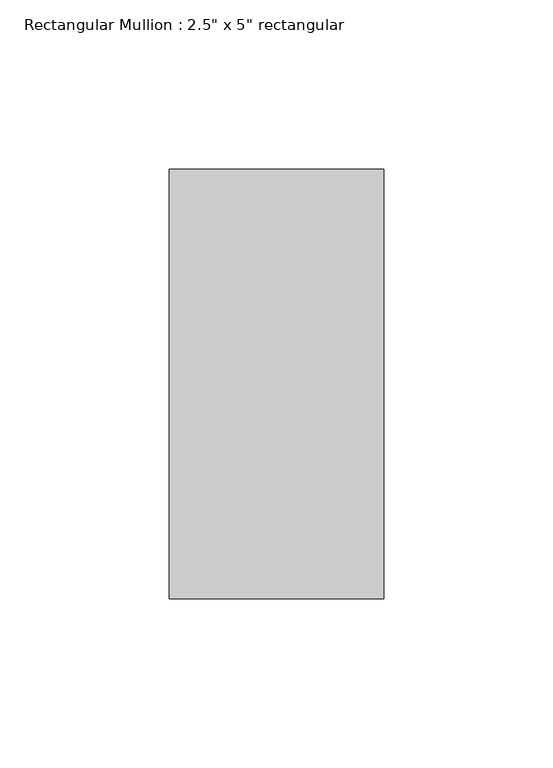
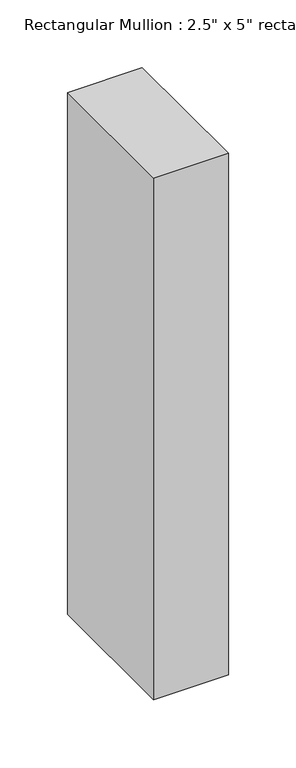
"""IFC4 building model written with IfcOpenShell, lengths in millimetres: member geometry."""

from ifc_helpers import new_model, si_unit, frame, origin, place, context, project, spatial, polyline, outline, extrude, source, transform, mapped, element, save


def member_9dc65bc2(model_context):
    return source(origin(), model_context, "Body", "SweptSolid", [
        extrude(outline(polyline([(0.0, 63.5), (0.0, -63.5), (-63.5, -63.5), (-63.5, 63.5), (0.0, 63.5)])), frame((0.0, 0.0, -469.9784063), z_axis=(0.0, 0.0, 1.0), x_axis=(1.0, 0.0, 0.0)), (0.0, 0.0, 1.0), 469.9784063),
    ])


if __name__ == "__main__":
    model = new_model("IFC4")
    model_context = context("Model", 3, world=origin())
    ifc_project = project(units=[si_unit("LENGTHUNIT", "METRE", prefix="MILLI")], contexts=[model_context])
    site = spatial("IfcSite", under=ifc_project)
    building = spatial("IfcBuilding", under=site)
    placement = place(None, origin())
    member_shape = member_9dc65bc2(model_context)
    element("IfcMember", 1, ObjectType="Rectangular Mullion : 2.5\" x 5\" rectangular", at=placement, inside=building, context=model_context, shape_type="MappedRepresentation", body=[
        mapped(member_shape, transform((0.0, 0.0, 0.0), x_axis=(1.0, 0.0, 0.0), y_axis=(0.0, 1.0, 0.0), z_axis=(0.0, 0.0, 1.0))),
    ])
    save(model, "model.ifc")

# Revit data of these elements
# Type "Rectangular Mullion : 2.5\" x 5\" rectangular"
#   built-in parameter 1007304 = 0.416667 (stored number, unit not read)
#   built-in parameter 1007301 = 0.104167 (stored number, unit not read)
#   built-in parameter 1007300 = 0.104167 (stored number, unit not read)
# Element 1 (IfcMember, "Rectangular Mullion : 2.5\" x 5\" rectangular")
#   Materials on its faces: "Aluminum"
# Materials
#   "Aluminum": class "Metal", colour RGB 247 247 247, transparency 0, Description = "Aluminum 6061", Cost = 0
